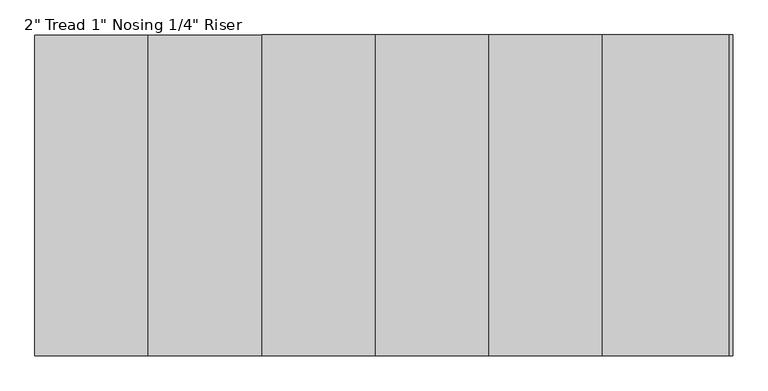
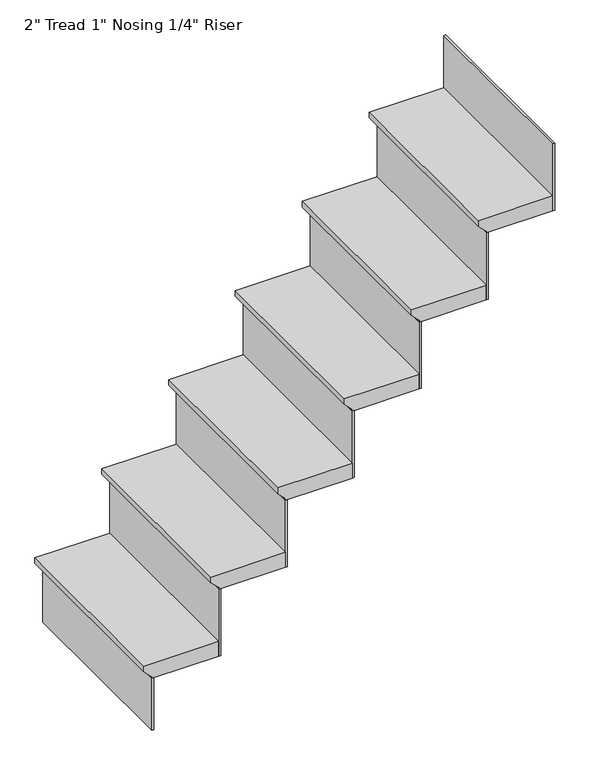
"""IFC4 building model written with IfcOpenShell, lengths in millimetres: stair flight geometry."""

from ifc_helpers import new_model, si_unit, origin, place, context, project, spatial, faceted_brep, source, transform, mapped, element, save


def stair_flight_d5a7a9e1(model_context):
    return source(origin(), model_context, "Body", "Brep", [
        faceted_brep([(-5028.1409298, -3848.0779636, 3409.95), (-5028.1409298, -3848.0779636, 3429.0), (-5028.1409298, -3238.4779636, 3429.0), (-5028.1409298, -3238.4779636, 3409.95), (-5002.7409298, -3848.0779636, 3384.55), (-5002.7409298, -3238.4779636, 3384.55), (-4786.8409298, -3848.0779636, 3429.0), (-4786.8409298, -3238.4779636, 3429.0), (-5002.7409298, -3238.4779636, 3378.2), (-4786.8409298, -3238.4779636, 3378.2), (-4786.8409298, -3848.0779636, 3378.2), (-5002.7409298, -3848.0779636, 3378.2)], [[[0, 1, 2, 3]], [[4, 0, 3, 5]], [[2, 1, 6, 7]], [[8, 9, 10, 11]], [[2, 7, 9, 8, 5, 3]], [[8, 11, 4, 5]], [[6, 1, 0, 4, 11, 10]], [[7, 6, 10, 9]]]),
        faceted_brep([(-5002.7409298, -3848.0779636, 3378.2), (-5002.7409298, -3848.0779636, 3200.4), (-4996.3909298, -3848.0779636, 3200.4), (-4996.3909298, -3848.0779636, 3378.2), (-5002.7409298, -3238.4779636, 3378.2), (-4996.3909298, -3238.4779636, 3378.2), (-4996.3909298, -3238.4779636, 3200.4), (-5002.7409298, -3238.4779636, 3200.4)], [[[0, 1, 2, 3]], [[4, 5, 6, 7]], [[1, 0, 4, 7]], [[2, 1, 7, 6]], [[3, 2, 6, 5]], [[0, 3, 5, 4]]]),
        faceted_brep([(-4786.8409298, -3848.0779636, 3606.8), (-4786.8409298, -3848.0779636, 3378.2), (-4780.4909298, -3848.0779636, 3378.2), (-4780.4909298, -3848.0779636, 3606.8), (-4786.8409298, -3238.4779636, 3606.8), (-4780.4909298, -3238.4779636, 3606.8), (-4780.4909298, -3238.4779636, 3378.2), (-4786.8409298, -3238.4779636, 3378.2)], [[[0, 1, 2, 3]], [[4, 5, 6, 7]], [[1, 0, 4, 7]], [[2, 1, 7, 6]], [[3, 2, 6, 5]], [[0, 3, 5, 4]]]),
        faceted_brep([(-4812.2409298, -3238.4779636, 3657.6), (-4812.2409298, -3848.0779636, 3657.6), (-4570.9409298, -3848.0779636, 3657.6), (-4570.9409298, -3238.4779636, 3657.6), (-4786.8409298, -3238.4779636, 3606.8), (-4570.9409298, -3238.4779636, 3606.8), (-4570.9409298, -3848.0779636, 3606.8), (-4786.8409298, -3848.0779636, 3606.8), (-4786.8409298, -3238.4779636, 3613.15), (-4812.2409298, -3238.4779636, 3638.55), (-4786.8409298, -3848.0779636, 3613.15), (-4812.2409298, -3848.0779636, 3638.55)], [[[0, 1, 2, 3]], [[4, 5, 6, 7]], [[0, 3, 5, 4, 8, 9]], [[4, 7, 10, 8]], [[2, 1, 11, 10, 7, 6]], [[3, 2, 6, 5]], [[11, 1, 0, 9]], [[10, 11, 9, 8]]]),
        faceted_brep([(-4570.9409298, -3848.0779636, 3835.4), (-4570.9409298, -3848.0779636, 3606.8), (-4564.5909298, -3848.0779636, 3606.8), (-4564.5909298, -3848.0779636, 3835.4), (-4570.9409298, -3238.4779636, 3835.4), (-4564.5909298, -3238.4779636, 3835.4), (-4564.5909298, -3238.4779636, 3606.8), (-4570.9409298, -3238.4779636, 3606.8)], [[[0, 1, 2, 3]], [[4, 5, 6, 7]], [[1, 0, 4, 7]], [[2, 1, 7, 6]], [[3, 2, 6, 5]], [[0, 3, 5, 4]]]),
        faceted_brep([(-4596.3409298, -3238.4779636, 3886.2), (-4596.3409298, -3848.0779636, 3886.2), (-4355.0409298, -3848.0779636, 3886.2), (-4355.0409298, -3238.4779636, 3886.2), (-4570.9409298, -3238.4779636, 3835.4), (-4355.0409298, -3238.4779636, 3835.4), (-4355.0409298, -3848.0779636, 3835.4), (-4570.9409298, -3848.0779636, 3835.4), (-4570.9409298, -3238.4779636, 3841.75), (-4596.3409298, -3238.4779636, 3867.15), (-4570.9409298, -3848.0779636, 3841.75), (-4596.3409298, -3848.0779636, 3867.15)], [[[0, 1, 2, 3]], [[4, 5, 6, 7]], [[0, 3, 5, 4, 8, 9]], [[4, 7, 10, 8]], [[2, 1, 11, 10, 7, 6]], [[3, 2, 6, 5]], [[11, 1, 0, 9]], [[10, 11, 9, 8]]]),
        faceted_brep([(-4355.0409298, -3848.0779636, 4064.0), (-4355.0409298, -3848.0779636, 3835.4), (-4348.6909298, -3848.0779636, 3835.4), (-4348.6909298, -3848.0779636, 4064.0), (-4355.0409298, -3238.4779636, 4064.0), (-4348.6909298, -3238.4779636, 4064.0), (-4348.6909298, -3238.4779636, 3835.4), (-4355.0409298, -3238.4779636, 3835.4)], [[[0, 1, 2, 3]], [[4, 5, 6, 7]], [[1, 0, 4, 7]], [[2, 1, 7, 6]], [[3, 2, 6, 5]], [[0, 3, 5, 4]]]),
        faceted_brep([(-4380.4409298, -3238.4779636, 4114.8), (-4380.4409298, -3848.0779636, 4114.8), (-4139.1409298, -3848.0779636, 4114.8), (-4139.1409298, -3238.4779636, 4114.8), (-4355.0409298, -3238.4779636, 4064.0), (-4139.1409298, -3238.4779636, 4064.0), (-4139.1409298, -3848.0779636, 4064.0), (-4355.0409298, -3848.0779636, 4064.0), (-4355.0409298, -3238.4779636, 4070.35), (-4380.4409298, -3238.4779636, 4095.75), (-4355.0409298, -3848.0779636, 4070.35), (-4380.4409298, -3848.0779636, 4095.75)], [[[0, 1, 2, 3]], [[4, 5, 6, 7]], [[0, 3, 5, 4, 8, 9]], [[4, 7, 10, 8]], [[2, 1, 11, 10, 7, 6]], [[3, 2, 6, 5]], [[11, 1, 0, 9]], [[10, 11, 9, 8]]]),
        faceted_brep([(-4139.1409298, -3848.0779636, 4292.6), (-4139.1409298, -3848.0779636, 4064.0), (-4132.7909298, -3848.0779636, 4064.0), (-4132.7909298, -3848.0779636, 4292.6), (-4139.1409298, -3238.4779636, 4292.6), (-4132.7909298, -3238.4779636, 4292.6), (-4132.7909298, -3238.4779636, 4064.0), (-4139.1409298, -3238.4779636, 4064.0)], [[[0, 1, 2, 3]], [[4, 5, 6, 7]], [[1, 0, 4, 7]], [[2, 1, 7, 6]], [[3, 2, 6, 5]], [[0, 3, 5, 4]]]),
        faceted_brep([(-4164.5409298, -3238.4779636, 4343.4), (-4164.5409298, -3848.0779636, 4343.4), (-3923.2409298, -3848.0779636, 4343.4), (-3923.2409298, -3238.4779636, 4343.4), (-4139.1409298, -3238.4779636, 4292.6), (-3923.2409298, -3238.4779636, 4292.6), (-3923.2409298, -3848.0779636, 4292.6), (-4139.1409298, -3848.0779636, 4292.6), (-4139.1409298, -3238.4779636, 4298.95), (-4164.5409298, -3238.4779636, 4324.35), (-4139.1409298, -3848.0779636, 4298.95), (-4164.5409298, -3848.0779636, 4324.35)], [[[0, 1, 2, 3]], [[4, 5, 6, 7]], [[0, 3, 5, 4, 8, 9]], [[4, 7, 10, 8]], [[2, 1, 11, 10, 7, 6]], [[3, 2, 6, 5]], [[11, 1, 0, 9]], [[10, 11, 9, 8]]]),
        faceted_brep([(-3707.3409298, -3848.0779636, 4749.8), (-3707.3409298, -3848.0779636, 4521.2), (-3700.9909298, -3848.0779636, 4521.2), (-3700.9909298, -3848.0779636, 4749.8), (-3707.3409298, -3238.4779636, 4749.8), (-3700.9909298, -3238.4779636, 4749.8), (-3700.9909298, -3238.4779636, 4521.2), (-3707.3409298, -3238.4779636, 4521.2)], [[[0, 1, 2, 3]], [[4, 5, 6, 7]], [[1, 0, 4, 7]], [[2, 1, 7, 6]], [[3, 2, 6, 5]], [[0, 3, 5, 4]]]),
        faceted_brep([(-3923.2409298, -3848.0779636, 4521.2), (-3923.2409298, -3848.0779636, 4292.6), (-3916.8909298, -3848.0779636, 4292.6), (-3916.8909298, -3848.0779636, 4521.2), (-3923.2409298, -3238.4779636, 4521.2), (-3916.8909298, -3238.4779636, 4521.2), (-3916.8909298, -3238.4779636, 4292.6), (-3923.2409298, -3238.4779636, 4292.6)], [[[0, 1, 2, 3]], [[4, 5, 6, 7]], [[1, 0, 4, 7]], [[2, 1, 7, 6]], [[3, 2, 6, 5]], [[0, 3, 5, 4]]]),
        faceted_brep([(-3707.3409298, -3238.4779636, 4572.0), (-3732.7409298, -3238.4779636, 4572.0), (-3948.6409298, -3238.4779636, 4572.0), (-3948.6409298, -3848.0779636, 4572.0), (-3707.3409298, -3848.0779636, 4572.0), (-3732.7409298, -3238.4779636, 4521.2), (-3707.3409298, -3238.4779636, 4521.2), (-3707.3409298, -3848.0779636, 4521.2), (-3923.2409298, -3848.0779636, 4521.2), (-3923.2409298, -3238.4779636, 4521.2), (-3923.2409298, -3238.4779636, 4527.55), (-3948.6409298, -3238.4779636, 4552.95), (-3923.2409298, -3848.0779636, 4527.55), (-3948.6409298, -3848.0779636, 4552.95)], [[[0, 1, 2, 3, 4]], [[5, 6, 7, 8, 9]], [[1, 0, 6, 5]], [[2, 1, 5, 9, 10, 11]], [[9, 8, 12, 10]], [[4, 3, 13, 12, 8, 7]], [[0, 4, 7, 6]], [[13, 3, 2, 11]], [[12, 13, 11, 10]]]),
    ])


if __name__ == "__main__":
    model = new_model("IFC4")
    model_context = context("Model", 3, world=origin())
    ifc_project = project(units=[si_unit("LENGTHUNIT", "METRE", prefix="MILLI")], contexts=[model_context])
    site = spatial("IfcSite", under=ifc_project)
    building = spatial("IfcBuilding", under=site)
    placement = place(None, origin())
    stair_flight_shape = stair_flight_d5a7a9e1(model_context)
    element("IfcStairFlight", 1, ObjectType="2\" Tread 1\" Nosing 1/4\" Riser", at=placement, inside=building, context=model_context, shape_type="MappedRepresentation", body=[
        mapped(stair_flight_shape, transform((0.0, 0.0, 0.0), x_axis=(1.0, 0.0, 0.0), y_axis=(0.0, 1.0, 0.0), z_axis=(0.0, 0.0, 1.0))),
    ])
    save(model, "model.ifc")
